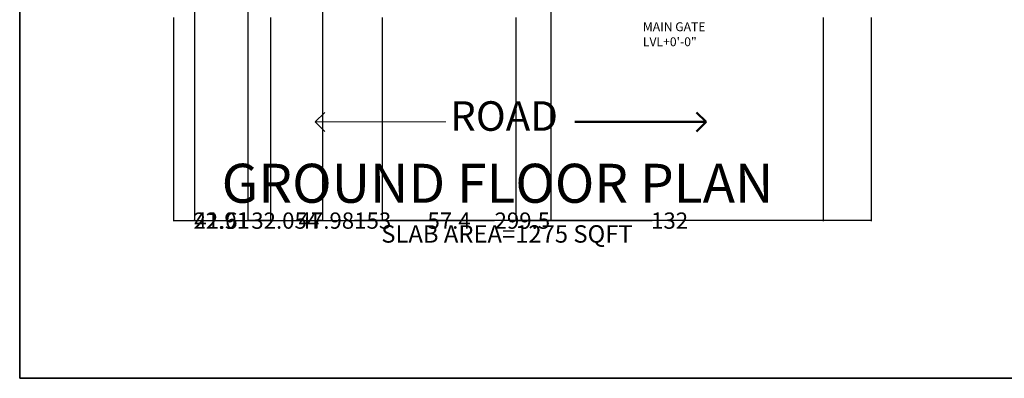
# Model space of a CAD drawing. Units: inches. Extents: x 1381 to 2246, y 1317 to 2168.
# Tile 1 of 15: x 1381 to 1804, y 1317 to 1471. Entities that reach past the tile are written whole.
import ezdxf

# ---------------------------------------------------------------- set-up
doc = ezdxf.new("R2010")
doc.units = ezdxf.units.IN
doc.header["$MEASUREMENT"] = 0
doc.layers.get('0').update_dxf_attribs({"color": 253})
for name, color, linetype, lineweight in [('A-ANNO-DIMS', 2, 'Continuous', 18), ('A-ANNO-SYMB', 7, 'Continuous', 18), ('A-ANNO-TEXT', 7, 'Continuous', 18), ('A-ANNO-TTLB', 7, 'Continuous', 35), ('A-AREA-IDEN', 3, 'Continuous', 25), ('A-WALL', 7, 'Continuous', 50)]:
    doc.layers.add(name, color=color, linetype=linetype, lineweight=lineweight)
doc.styles.get("Standard").update_dxf_attribs({"font": 'arial.ttf'})
doc.dimstyles.get("Standard").update_dxf_attribs({"dimtxt": 7, "dimasz": 0.18, "dimexe": 0.18, "dimexo": 0.0625, "dimgap": 0.09, "dimtad": 0, "dimtih": 1, "dimtoh": 1, "dimdec": 1, "dimzin": 0, "dimdsep": 46, "dimlunit": 3, "dimtxsty": 'Standard', "dimcen": 0.09, "dimadec": 0, "dimazin": 0, "dimtfac": 1, "dimtdec": 1, "dimtofl": 0, "dimtmove": 0, "dimatfit": 3, "dimfxl": 1, "dimtolj": 1, "dimtzin": 0, "dimarcsym": 0})

# ---------------------------------------------------------------- blocks, each defined once
blk = doc.blocks.new('ARROW-ROAD')
for q in [(4.11, 8.25), (56.05, 4.15), (4.15, 0)]:
    blk.add_line((0, 4.15), q)
blk = doc.blocks.new('*D49')
at = {"layer": 'A-ANNO-DIMS', "color": 0, "lineweight": -2, "transparency": 16777216}
for p, q in [((1447.05, 1471.85), (1447.05, 1384.36)), ((1746.55, 1471.85), (1746.55, 1384.36)), ((1447.23, 1384.54), (1584.81, 1384.54)), ((1746.37, 1384.54), (1608.79, 1384.54))]:
    blk.add_line(p, q, dxfattribs=at)
at = {"layer": 'A-ANNO-DIMS', "color": 0, "transparency": 16777216}
for points in [[(1447.23, 1384.57), (1447.23, 1384.51), (1447.05, 1384.54)], [(1746.37, 1384.57), (1746.37, 1384.51), (1746.55, 1384.54)]]:
    blk.add_solid(points, dxfattribs=at)
at = {"layer": 'Defpoints', "color": 0, "transparency": 16777216}
for p in [(1447.05, 1471.92), (1746.55, 1471.92), (1746.55, 1384.54)]:
    blk.add_point(p, dxfattribs=at)
at = {"layer": 'A-ANNO-DIMS', "color": 0, "transparency": 16777216, "insert": (1596.8, 1384.54), "char_height": 7, "attachment_point": 5}
blk.add_mtext('\\A1;299.5', dxfattribs=at)
blk = doc.blocks.new('*D62')
at = {"layer": 'A-ANNO-DIMS', "color": 0, "lineweight": -2, "transparency": 16777216}
for p, q in [((1447.05, 1471.85), (1447.05, 1384.36)), ((1488.66, 1471.85), (1488.66, 1384.36)), ((1447.23, 1384.54), (1456.49, 1384.54)), ((1488.48, 1384.54), (1479.22, 1384.54))]:
    blk.add_line(p, q, dxfattribs=at)
at = {"layer": 'A-ANNO-DIMS', "color": 0, "transparency": 16777216}
for points in [[(1447.23, 1384.57), (1447.23, 1384.51), (1447.05, 1384.54)], [(1488.48, 1384.57), (1488.48, 1384.51), (1488.66, 1384.54)]]:
    blk.add_solid(points, dxfattribs=at)
at = {"layer": 'Defpoints', "color": 0, "transparency": 16777216}
for p in [(1447.05, 1471.92), (1488.66, 1471.92), (1488.66, 1384.54)]:
    blk.add_point(p, dxfattribs=at)
at = {"layer": 'A-ANNO-DIMS', "color": 0, "transparency": 16777216, "insert": (1467.86, 1384.54), "char_height": 7, "attachment_point": 5}
blk.add_mtext('\\A1;41.61', dxfattribs=at)
blk = doc.blocks.new('*D63')
at = {"layer": 'A-ANNO-DIMS', "color": 0, "lineweight": -2, "transparency": 16777216}
for p, q in [((1488.66, 1471.85), (1488.66, 1384.36)), ((1536.65, 1471.85), (1536.65, 1384.36)), ((1488.84, 1384.54), (1500.61, 1384.54)), ((1536.47, 1384.54), (1524.7, 1384.54))]:
    blk.add_line(p, q, dxfattribs=at)
at = {"layer": 'A-ANNO-DIMS', "color": 0, "transparency": 16777216}
for points in [[(1488.84, 1384.57), (1488.84, 1384.51), (1488.66, 1384.54)], [(1536.47, 1384.57), (1536.47, 1384.51), (1536.65, 1384.54)]]:
    blk.add_solid(points, dxfattribs=at)
at = {"layer": 'Defpoints', "color": 0, "transparency": 16777216}
for p in [(1488.66, 1471.92), (1536.65, 1471.92), (1536.65, 1384.54)]:
    blk.add_point(p, dxfattribs=at)
at = {"layer": 'A-ANNO-DIMS', "color": 0, "transparency": 16777216, "insert": (1512.65, 1384.54), "char_height": 7, "attachment_point": 5}
blk.add_mtext('\\A1;47.98', dxfattribs=at)
blk = doc.blocks.new('*D64')
at = {"layer": 'A-ANNO-DIMS', "color": 0, "lineweight": -2, "transparency": 16777216}
for p, q in [((1536.65, 1471.85), (1536.65, 1384.36)), ((1594.05, 1471.85), (1594.05, 1384.36)), ((1536.83, 1384.54), (1556.18, 1384.54)), ((1593.87, 1384.54), (1574.51, 1384.54))]:
    blk.add_line(p, q, dxfattribs=at)
at = {"layer": 'A-ANNO-DIMS', "color": 0, "transparency": 16777216}
for points in [[(1536.83, 1384.57), (1536.83, 1384.51), (1536.65, 1384.54)], [(1593.87, 1384.57), (1593.87, 1384.51), (1594.05, 1384.54)]]:
    blk.add_solid(points, dxfattribs=at)
at = {"layer": 'Defpoints', "color": 0, "transparency": 16777216}
for p in [(1536.65, 1471.92), (1594.05, 1471.92), (1594.05, 1384.54)]:
    blk.add_point(p, dxfattribs=at)
at = {"layer": 'A-ANNO-DIMS', "color": 0, "transparency": 16777216, "insert": (1565.35, 1384.54), "char_height": 7, "attachment_point": 5}
blk.add_mtext('\\A1;57.4', dxfattribs=at)
blk = doc.blocks.new('*D65')
at = {"layer": 'A-ANNO-DIMS', "color": 0, "lineweight": -2, "transparency": 16777216}
for p, q in [((1594.05, 1471.85), (1594.05, 1384.36)), ((1726.05, 1471.85), (1726.05, 1384.36)), ((1594.23, 1384.54), (1652.59, 1384.54)), ((1725.87, 1384.54), (1667.5, 1384.54))]:
    blk.add_line(p, q, dxfattribs=at)
at = {"layer": 'A-ANNO-DIMS', "color": 0, "transparency": 16777216}
for points in [[(1594.23, 1384.57), (1594.23, 1384.51), (1594.05, 1384.54)], [(1725.87, 1384.57), (1725.87, 1384.51), (1726.05, 1384.54)]]:
    blk.add_solid(points, dxfattribs=at)
at = {"layer": 'Defpoints', "color": 0, "transparency": 16777216}
for p in [(1594.05, 1471.92), (1726.05, 1471.92), (1726.05, 1384.54)]:
    blk.add_point(p, dxfattribs=at)
at = {"layer": 'A-ANNO-DIMS', "color": 0, "transparency": 16777216, "insert": (1660.05, 1384.54), "char_height": 7, "attachment_point": 5}
blk.add_mtext('\\A1;132', dxfattribs=at)
blk = doc.blocks.new('*D66')
at = {"layer": 'A-ANNO-DIMS', "color": 0, "lineweight": -2, "transparency": 16777216}
for p, q in [((1456.05, 1578.35), (1456.05, 1384.36)), ((1609.05, 1578.35), (1609.05, 1384.36)), ((1456.23, 1384.54), (1525.06, 1384.54)), ((1608.87, 1384.54), (1540.04, 1384.54))]:
    blk.add_line(p, q, dxfattribs=at)
at = {"layer": 'A-ANNO-DIMS', "color": 0, "transparency": 16777216}
for points in [[(1456.23, 1384.57), (1456.23, 1384.51), (1456.05, 1384.54)], [(1608.87, 1384.57), (1608.87, 1384.51), (1609.05, 1384.54)]]:
    blk.add_solid(points, dxfattribs=at)
at = {"layer": 'Defpoints', "color": 0, "transparency": 16777216}
for p in [(1456.05, 1578.42), (1609.05, 1578.42), (1609.05, 1384.54)]:
    blk.add_point(p, dxfattribs=at)
at = {"layer": 'A-ANNO-DIMS', "color": 0, "transparency": 16777216, "insert": (1532.55, 1384.54), "char_height": 7, "attachment_point": 5}
blk.add_mtext('\\A1;153', dxfattribs=at)
blk = doc.blocks.new('*D67')
at = {"layer": 'A-ANNO-DIMS', "color": 0, "lineweight": -2, "transparency": 16777216}
for p, q in [((1456.050973, 1911.353813), (1456.050973, 1384.360695)), ((1478.962127, 1911.353813), (1478.962127, 1384.360695)), ((1455.870973, 1384.540695), (1455.690973, 1384.540695)), ((1479.142127, 1384.540695), (1479.322127, 1384.540695))]:
    blk.add_line(p, q, dxfattribs=at)
at = {"layer": 'A-ANNO-DIMS', "color": 0, "transparency": 16777216}
for points in [[(1455.870973, 1384.570695), (1455.870973, 1384.510695), (1456.050973, 1384.540695)], [(1479.142127, 1384.570695), (1479.142127, 1384.510695), (1478.962127, 1384.540695)]]:
    blk.add_solid(points, dxfattribs=at)
at = {"layer": 'Defpoints', "color": 0, "transparency": 16777216}
for p in [(1456.050973, 1911.416313), (1478.962127, 1911.416313), (1478.962127, 1384.540695)]:
    blk.add_point(p, dxfattribs=at)
at = {"layer": 'A-ANNO-DIMS', "color": 0, "transparency": 16777216, "insert": (1467.50655, 1384.540695), "char_height": 7, "attachment_point": 5}
blk.add_mtext('\\A1;22.91', dxfattribs=at)
blk = doc.blocks.new('*D68')
at = {"layer": 'A-ANNO-DIMS', "color": 0, "lineweight": -2, "transparency": 16777216}
for p, q in [((1478.96, 1911.35), (1478.96, 1384.36)), ((1511.02, 1911.35), (1511.02, 1384.36)), ((1479.14, 1384.54), (1480.39, 1384.54)), ((1510.84, 1384.54), (1509.59, 1384.54))]:
    blk.add_line(p, q, dxfattribs=at)
at = {"layer": 'A-ANNO-DIMS', "color": 0, "transparency": 16777216}
for points in [[(1479.14, 1384.57), (1479.14, 1384.51), (1478.96, 1384.54)], [(1510.84, 1384.57), (1510.84, 1384.51), (1511.02, 1384.54)]]:
    blk.add_solid(points, dxfattribs=at)
at = {"layer": 'Defpoints', "color": 0, "transparency": 16777216}
for p in [(1478.96, 1911.42), (1511.02, 1911.42), (1511.02, 1384.54)]:
    blk.add_point(p, dxfattribs=at)
at = {"layer": 'A-ANNO-DIMS', "color": 0, "transparency": 16777216, "insert": (1494.99, 1384.54), "char_height": 7, "attachment_point": 5}
blk.add_mtext('\\A1;32.054', dxfattribs=at)

msp = doc.modelspace()

# ---------------------------------------------------------------- linework, layer by layer
at = {"layer": 'A-ANNO-TTLB'}
for p, q in [((1380.9518, 1316.7761), (1380.9518, 2167.8236)), ((2244.072, 1316.7761), (1380.9518, 1316.7761))]:
    msp.add_line(p, q, dxfattribs=at)
at = {"layer": 'A-WALL'}
for p, q in [((1675.6941, 1426.938), (1671.5842, 1431.0452)), ((1619.3958, 1426.938), (1675.6941, 1426.938)), ((1675.6941, 1426.938), (1671.5495, 1422.7907))]:
    msp.add_line(p, q, dxfattribs=at)

# ---------------------------------------------------------------- block references
at = {"layer": 'A-ANNO-SYMB'}
msp.add_blockref('ARROW-ROAD', (1507.898, 1422.791), dxfattribs=at)

# ---------------------------------------------------------------- texts
at = {"layer": 'A-ANNO-TEXT'}
for s, height, p in [('MAIN GATE', 3.83139, (1648.5671, 1465.93)), ('LVL+0\'-0"', 3.83139, (1648.5671, 1459.4668)), ('ROAD', 12.68973, (1565.8393, 1423.1241)), ('SLAB AREA=1275 SQFT', 7.495394, (1536.2348, 1375.0646))]:
    msp.add_text(s, height=height, dxfattribs=at).set_placement(p)
at = {"layer": 'A-AREA-IDEN'}
msp.add_text('GROUND FLOOR PLAN', height=16.755681, dxfattribs=at).set_placement((1467.6968, 1392.2038))

# ---------------------------------------------------------------- dimensions: what is measured, and where the dimension line sits
at = {"layer": 'A-ANNO-DIMS'}
for base, p1, p2, override, picture, middle in [((1478.9621, 1384.5407), (1456.051, 1911.4163), (1478.9621, 1911.4163), {"dimdec": 2, "dimlfac": 1, "dimrnd": 0, "dimzin": 0, "dimdsep": 46, "dimlunit": 2}, '*D67', (1467.5066, 1384.5407)), ((1511.016, 1384.5407), (1478.9621, 1911.4163), (1511.016, 1911.4163), {"dimdec": 3, "dimlfac": 1, "dimrnd": 0, "dimzin": 0, "dimdsep": 46, "dimlunit": 2}, '*D68', (1494.9891, 1384.5407)), ((1609.051, 1384.5407), (1456.051, 1578.4163), (1609.051, 1578.4163), {"dimdec": 0, "dimlfac": 1, "dimrnd": 0, "dimzin": 0, "dimdsep": 46, "dimlunit": 2}, '*D66', (1532.551, 1384.5407)), ((1746.551, 1384.5407), (1447.051, 1471.9163), (1746.551, 1471.9163), {"dimdec": 1, "dimlfac": 1, "dimrnd": 0, "dimzin": 0, "dimdsep": 46, "dimlunit": 2}, '*D49', (1596.801, 1384.5407)), ((1488.6632, 1384.5407), (1447.051, 1471.9163), (1488.6632, 1471.9163), {"dimdec": 2, "dimlfac": 1, "dimrnd": 0, "dimzin": 0, "dimdsep": 46, "dimlunit": 2}, '*D62', (1467.8571, 1384.5407)), ((1536.6467, 1384.5407), (1488.6632, 1471.9163), (1536.6467, 1471.9163), {"dimdec": 2, "dimlfac": 1, "dimrnd": 0, "dimzin": 0, "dimdsep": 46, "dimlunit": 2}, '*D63', (1512.655, 1384.5407)), ((1594.0453, 1384.5407), (1536.6467, 1471.9163), (1594.0453, 1471.9163), {"dimdec": 1, "dimlfac": 1, "dimrnd": 0, "dimzin": 0, "dimdsep": 46, "dimlunit": 2}, '*D64', (1565.346, 1384.5407)), ((1726.0453, 1384.5407), (1594.0453, 1471.9163), (1726.0453, 1471.9163), {"dimdec": 0, "dimlfac": 1, "dimrnd": 0, "dimzin": 0, "dimdsep": 46, "dimlunit": 2}, '*D65', (1660.0453, 1384.5407))]:
    dim = msp.add_linear_dim(base=base, p1=p1, p2=p2, dimstyle='Standard', override=override, dxfattribs=at)
    dim.commit()
    dim.dimension.update_dxf_attribs({"geometry": picture, "text_midpoint": middle})

doc.saveas('drawing.dxf')
